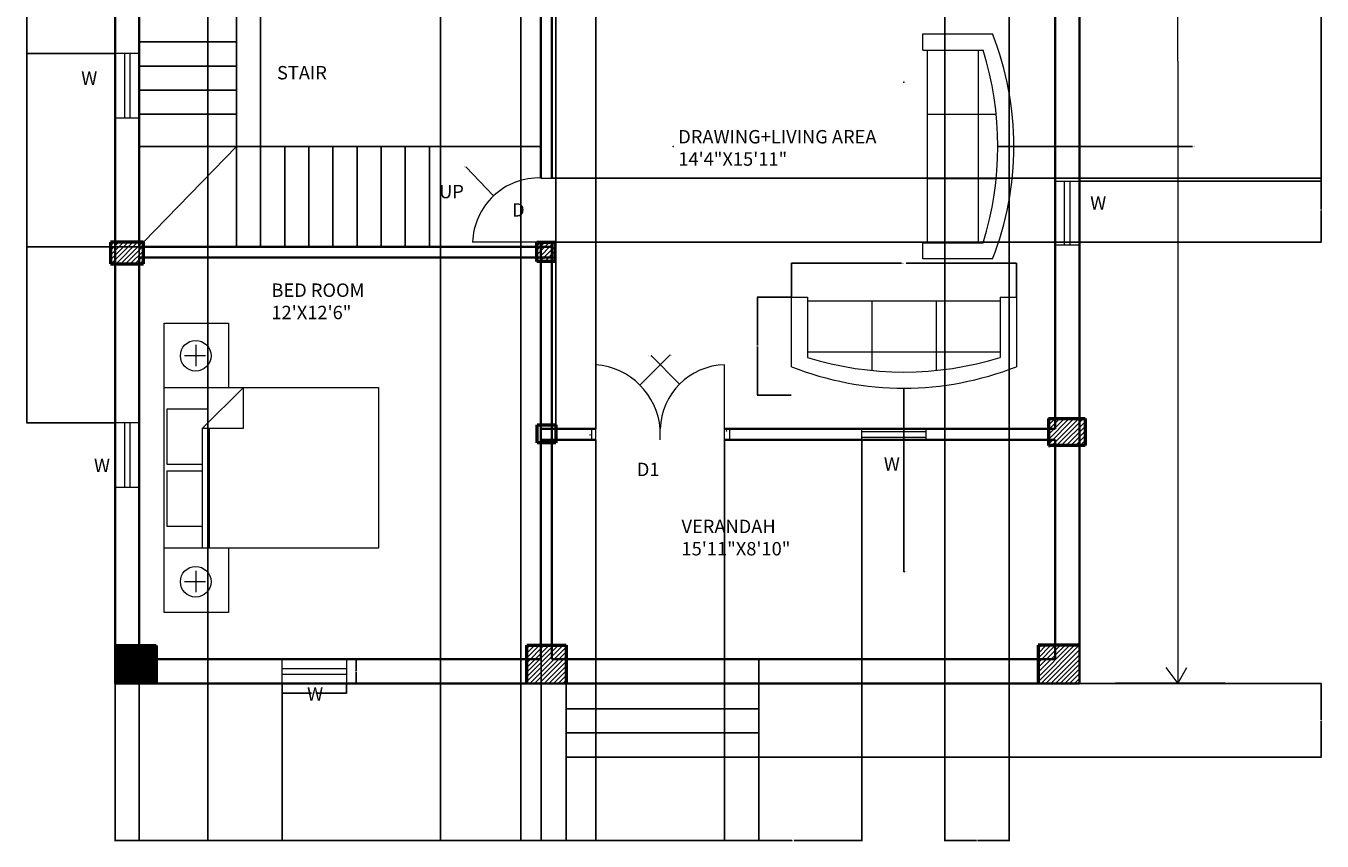
# Model space of a CAD drawing. Units: inches. Extents: x -12 to 472, y -585 to 99.
# Tile 1 of 4: x -12 to 472, y -585 to -281. Entities that reach past the tile are written whole.
import ezdxf

# ---------------------------------------------------------------- set-up
doc = ezdxf.new("R2010")
doc.units = ezdxf.units.IN
doc.header["$MEASUREMENT"] = 0
for name, color, linetype, lineweight in [('A-ANNO-DIMS', 2, 'Continuous', 18), ('A-ANNO-TEXT', 7, 'Continuous', 18), ('A-AREA-IDEN', 7, 'Continuous', 25), ('A-COLS', 7, 'Continuous', 50), ('A-COLS-PATT', 252, 'Continuous', 13), ('A-DOOR', 3, 'Continuous', 18), ('A-FLOR-STRS', 7, 'Continuous', 25), ('A-FURN', 8, 'Continuous', 18), ('A-GLAZ', 4, 'Continuous', 18), ('A-WALL', 7, 'Continuous', 35)]:
    doc.layers.add(name, color=color, linetype=linetype, lineweight=lineweight)
doc.styles.get("Standard").update_dxf_attribs({"font": 'arial.ttf'})
doc.dimstyles.get("Standard").update_dxf_attribs({"dimtxt": 0.18, "dimasz": 0.18, "dimexe": 0.18, "dimexo": 0.0625, "dimgap": 0.09, "dimtad": 0, "dimtih": 1, "dimtoh": 1, "dimdec": 4, "dimzin": 0, "dimdsep": 46, "dimtxsty": 'Standard', "dimcen": 0.09, "dimadec": 0, "dimazin": 0, "dimtfac": 1, "dimtdec": 4, "dimtofl": 0, "dimtmove": 0, "dimatfit": 3, "dimfxl": 1, "dimtolj": 1, "dimtzin": 0, "dimarcsym": 0})
pattern_1 = [(45, (-1281.9002, -702.7604), (-0.8838835, 0.8838835), [])]

# ---------------------------------------------------------------- blocks, each defined once
blk = doc.blocks.new('Bed - Queen')
for p, q in [((0, -80.00003), (0, 0)), ((0, 0), (59.99999, 0)), ((59.99999, 0), (59.99999, -80.00003)), ((7.99999, -1.2), (28.79998, -1.2)), ((7.99999, -14.4), (7.99999, -1.2)), ((28.79998, -1.2), (28.79998, -14.4)), ((31.19999, -1.2), (51.99999, -1.2)), ((31.19999, -14.4), (31.19999, -1.2)), ((51.99999, -1.2), (51.99999, -16.4)), ((0, -14.4), (44.8, -14.4)), ((59.99999, -29.6), (44.8, -14.4)), ((44.8, -14.4), (44.8, -29.6)), ((44.8, -16.8), (0, -16.8)), ((51.99999, -16.4), (46.79936, -16.4)), ((44.8, -29.6), (59.99999, -29.6)), ((59.99999, -80.00003), (0, -80.00003))]:
    blk.add_line(p, q)
blk = doc.blocks.new('Sofa - Roundback 7 ft.')
for p, q in [((-12.00002, -32.4421), (-12.00003, -6.5971)), ((11.99997, -32.4421), (11.99998, -6.5971)), ((-36.000027, -34), (-36.000027, -11.4696)), ((-35.999844, -13.3819), (35.9998, -13.3819)), ((35.99998, -34), (35.99998, -11.4696)), ((-36.000027, -32.4421), (35.99998, -32.4421))]:
    blk.add_line(p, q)
for points in [[(-36.000027, -34), (-42.000027, -34), (-42.000027, -8)], [(41.99998, -8), (41.99998, -34), (35.99998, -34)]]:
    blk.add_lwpolyline(points)
for centre, radius, start, end in [((0, -114.25), 114.25, 68.43141, 111.5686), ((-0.00001, -127.1968), 121.1968, 72.72033, 107.2797)]:
    blk.add_arc(centre, radius, start, end)
blk = doc.blocks.new('WIN-24IN-EXT')
for p, q in [((0, 5.5), (24, 5.5)), ((0, 3.5), (24, 3.5))]:
    blk.add_line(p, q)
blk.add_lwpolyline([(0, 9), (24, 9), (24, 0), (0, 0)], close=True)
blk = doc.blocks.new('NIGHTSTAND-24IN')
for p, q in [((0, 24), (24, 24)), ((24, 24), (24, 0)), ((24, 0), (0, 0))]:
    blk.add_line(p, q)
blk = doc.blocks.new('LAMP-BEDSIDE-PLAN')
for p, q in [((5.72, 9.81), (5.72, 1.79)), ((1.49, 5.8), (9.4, 5.8))]:
    blk.add_line(p, q)
blk.add_circle((5.72, 5.72), 5.72)
blk = doc.blocks.new('*D10')
at = {"layer": 'A-ANNO-DIMS', "color": 0, "lineweight": -2, "transparency": 16777216}
for p, q in [((83.68, -526.44), (83.68, -530.16)), ((107.68, -526.44), (107.68, -530.16)), ((83.86, -529.98), (94.57, -529.98)), ((107.5, -529.98), (96.8, -529.98))]:
    blk.add_line(p, q, dxfattribs=at)
at = {"layer": 'A-ANNO-DIMS', "color": 0, "transparency": 16777216}
for points in [[(83.86, -529.95), (83.86, -530.01), (83.68, -529.98)], [(107.5, -529.95), (107.5, -530.01), (107.68, -529.98)]]:
    blk.add_solid(points, dxfattribs=at)
at = {"layer": 'Defpoints', "color": 0, "transparency": 16777216}
for p in [(83.68, -526.38), (107.68, -526.38), (107.68, -529.98)]:
    blk.add_point(p, dxfattribs=at)
at = {"layer": 'A-ANNO-DIMS', "color": 0, "transparency": 16777216, "insert": (95.68, -529.98), "char_height": 0.18, "attachment_point": 5}
blk.add_mtext('\\A1;WINDOW 24 TYP.', dxfattribs=at)
blk = doc.blocks.new('*D11')
at = {"layer": 'A-ANNO-DIMS', "color": 0, "lineweight": -2, "transparency": 16777216}
for p, q in [((107.75, -517.38), (111.46, -517.38)), ((111.28, -517.56), (111.28, -521.7)), ((111.28, -526.2), (111.28, -522.06)), ((107.75, -526.38), (111.46, -526.38))]:
    blk.add_line(p, q, dxfattribs=at)
at = {"layer": 'A-ANNO-DIMS', "color": 0, "transparency": 16777216}
for points in [[(111.25, -517.56), (111.31, -517.56), (111.28, -517.38)], [(111.25, -526.2), (111.31, -526.2), (111.28, -526.38)]]:
    blk.add_solid(points, dxfattribs=at)
at = {"layer": 'Defpoints', "color": 0, "transparency": 16777216}
for p in [(107.68, -517.38), (111.28, -517.38), (107.68, -526.38)]:
    blk.add_point(p, dxfattribs=at)
at = {"layer": 'A-ANNO-DIMS', "color": 0, "transparency": 16777216, "insert": (111.28, -521.88), "char_height": 0.18, "attachment_point": 5}
blk.add_mtext('\\A1;9 TYP.', dxfattribs=at)
blk = doc.blocks.new('*D22')
at = {"layer": 'A-ANNO-DIMS', "color": 0, "lineweight": -2, "transparency": 16777216}
for p, q in [((273.76, -382.06), (273.76, -369.34)), ((273.94, -369.52), (314.86, -369.52)), ((357.58, -369.52), (316.67, -369.52)), ((357.76, -382.06), (357.76, -369.34))]:
    blk.add_line(p, q, dxfattribs=at)
at = {"layer": 'A-ANNO-DIMS', "color": 0, "transparency": 16777216}
for points in [[(273.94, -369.49), (273.94, -369.55), (273.76, -369.52)], [(357.58, -369.49), (357.58, -369.55), (357.76, -369.52)]]:
    blk.add_solid(points, dxfattribs=at)
at = {"layer": 'Defpoints', "color": 0, "transparency": 16777216}
for p in [(273.76, -369.52), (273.76, -382.12), (357.76, -382.12)]:
    blk.add_point(p, dxfattribs=at)
at = {"layer": 'A-ANNO-DIMS', "color": 0, "transparency": 16777216, "insert": (315.76, -369.52), "char_height": 0.18, "attachment_point": 5}
blk.add_mtext('\\A1;SOFA 84 TYP.', dxfattribs=at)
blk = doc.blocks.new('*D23')
at = {"layer": 'A-ANNO-DIMS', "color": 0, "lineweight": -2, "transparency": 16777216}
for p, q in [((273.7, -382.12), (260.98, -382.12)), ((261.16, -382.3), (261.16, -400.27)), ((261.16, -418.61), (261.16, -400.64)), ((273.7, -418.79), (260.98, -418.79))]:
    blk.add_line(p, q, dxfattribs=at)
at = {"layer": 'A-ANNO-DIMS', "color": 0, "transparency": 16777216}
for points in [[(261.13, -382.3), (261.19, -382.3), (261.16, -382.12)], [(261.13, -418.61), (261.19, -418.61), (261.16, -418.79)]]:
    blk.add_solid(points, dxfattribs=at)
at = {"layer": 'Defpoints', "color": 0, "transparency": 16777216}
for p in [(273.76, -382.12), (261.16, -418.79), (273.76, -418.79)]:
    blk.add_point(p, dxfattribs=at)
at = {"layer": 'A-ANNO-DIMS', "color": 0, "transparency": 16777216, "insert": (261.16, -400.46), "char_height": 0.18, "attachment_point": 5}
blk.add_mtext('\\A1;37 TYP.', dxfattribs=at)
blk = doc.blocks.new('*D26')
at = {"layer": 'A-ANNO-DIMS', "color": 0, "lineweight": -2, "transparency": 16777216}
for p, q in [((21.28, -526.44), (21.28, -585.26)), ((83.68, -526.44), (83.68, -585.26)), ((21.46, -585.08), (52.16, -585.08)), ((83.5, -585.08), (52.8, -585.08))]:
    blk.add_line(p, q, dxfattribs=at)
at = {"layer": 'A-ANNO-DIMS', "color": 0, "transparency": 16777216}
for points in [[(21.46, -585.05), (21.46, -585.11), (21.28, -585.08)], [(83.5, -585.05), (83.5, -585.11), (83.68, -585.08)]]:
    blk.add_solid(points, dxfattribs=at)
at = {"layer": 'Defpoints', "color": 0, "transparency": 16777216}
for p in [(21.28, -526.38), (83.68, -526.38), (83.68, -585.08)]:
    blk.add_point(p, dxfattribs=at)
at = {"layer": 'A-ANNO-DIMS', "color": 0, "transparency": 16777216, "insert": (52.48, -585.08), "char_height": 0.18, "attachment_point": 5}
blk.add_mtext('\\A1;62.4', dxfattribs=at)
blk = doc.blocks.new('*D27')
at = {"layer": 'A-ANNO-DIMS', "color": 0, "lineweight": -2, "transparency": 16777216}
for p, q in [((83.68, -526.44), (83.68, -585.26)), ((189.63, -553.94), (189.63, -585.26)), ((83.86, -585.08), (136.2, -585.08)), ((189.45, -585.08), (137.12, -585.08))]:
    blk.add_line(p, q, dxfattribs=at)
at = {"layer": 'A-ANNO-DIMS', "color": 0, "transparency": 16777216}
for points in [[(83.86, -585.05), (83.86, -585.11), (83.68, -585.08)], [(189.45, -585.05), (189.45, -585.11), (189.63, -585.08)]]:
    blk.add_solid(points, dxfattribs=at)
at = {"layer": 'Defpoints', "color": 0, "transparency": 16777216}
for p in [(83.68, -526.38), (189.63, -553.88), (189.63, -585.08)]:
    blk.add_point(p, dxfattribs=at)
at = {"layer": 'A-ANNO-DIMS', "color": 0, "transparency": 16777216, "insert": (136.66, -585.08), "char_height": 0.18, "attachment_point": 5}
blk.add_mtext('\\A1;105.95', dxfattribs=at)
blk = doc.blocks.new('*D28')
at = {"layer": 'A-ANNO-DIMS', "color": 0, "lineweight": -2, "transparency": 16777216}
for p, q in [((189.63, -553.94), (189.63, -585.26)), ((261.62, -553.94), (261.62, -585.26)), ((189.81, -585.08), (225.23, -585.08)), ((261.44, -585.08), (226.02, -585.08))]:
    blk.add_line(p, q, dxfattribs=at)
at = {"layer": 'A-ANNO-DIMS', "color": 0, "transparency": 16777216}
for points in [[(189.81, -585.05), (189.81, -585.11), (189.63, -585.08)], [(261.44, -585.05), (261.44, -585.11), (261.62, -585.08)]]:
    blk.add_solid(points, dxfattribs=at)
at = {"layer": 'Defpoints', "color": 0, "transparency": 16777216}
for p in [(189.63, -553.88), (261.62, -553.88), (261.62, -585.08)]:
    blk.add_point(p, dxfattribs=at)
at = {"layer": 'A-ANNO-DIMS', "color": 0, "transparency": 16777216, "insert": (225.63, -585.08), "char_height": 0.18, "attachment_point": 5}
blk.add_mtext('\\A1;71.98', dxfattribs=at)
blk = doc.blocks.new('*D29')
at = {"layer": 'A-ANNO-DIMS', "color": 0, "lineweight": -2, "transparency": 16777216}
for p, q in [((381.34, -526.38), (471.69, -526.38)), ((471.51, -526.56), (471.51, -539.95)), ((471.51, -553.7), (471.51, -540.31)), ((261.68, -553.88), (471.69, -553.88))]:
    blk.add_line(p, q, dxfattribs=at)
at = {"layer": 'A-ANNO-DIMS', "color": 0, "transparency": 16777216}
for points in [[(471.48, -526.56), (471.54, -526.56), (471.51, -526.38)], [(471.48, -553.7), (471.54, -553.7), (471.51, -553.88)]]:
    blk.add_solid(points, dxfattribs=at)
at = {"layer": 'Defpoints', "color": 0, "transparency": 16777216}
for p in [(381.28, -526.38), (471.51, -526.38), (261.62, -553.88)]:
    blk.add_point(p, dxfattribs=at)
at = {"layer": 'A-ANNO-DIMS', "color": 0, "transparency": 16777216, "insert": (471.51, -540.13), "char_height": 0.18, "attachment_point": 5}
blk.add_mtext('\\A1;27.5', dxfattribs=at)
blk = doc.blocks.new('*D30')
at = {"layer": 'A-ANNO-DIMS', "color": 0, "lineweight": -2, "transparency": 16777216}
for p, q in [((185.8, -429.83), (185.8, 98.81)), ((185.98, 98.63), (193.09, 98.63)), ((200.62, 98.63), (193.51, 98.63)), ((200.8, -431.32), (200.8, 98.81))]:
    blk.add_line(p, q, dxfattribs=at)
at = {"layer": 'A-ANNO-DIMS', "color": 0, "transparency": 16777216}
for points in [[(185.98, 98.66), (185.98, 98.6), (185.8, 98.63)], [(200.62, 98.66), (200.62, 98.6), (200.8, 98.63)]]:
    blk.add_solid(points, dxfattribs=at)
at = {"layer": 'Defpoints', "color": 0, "transparency": 16777216}
for p in [(200.8, 98.63), (185.8, -429.9), (200.8, -431.38)]:
    blk.add_point(p, dxfattribs=at)
at = {"layer": 'A-ANNO-DIMS', "color": 0, "transparency": 16777216, "insert": (193.3, 98.63), "char_height": 0.18, "attachment_point": 5}
blk.add_mtext('\\A1;15', dxfattribs=at)
blk = doc.blocks.new('*D31')
at = {"layer": 'A-ANNO-DIMS', "color": 0, "lineweight": -2, "transparency": 16777216}
for p, q in [((200.8, -435.44), (200.8, -585.26)), ((248.8, -435.44), (248.8, -585.26)), ((200.98, -585.08), (224.58, -585.08)), ((248.62, -585.08), (225.03, -585.08))]:
    blk.add_line(p, q, dxfattribs=at)
at = {"layer": 'A-ANNO-DIMS', "color": 0, "transparency": 16777216}
for points in [[(200.98, -585.05), (200.98, -585.11), (200.8, -585.08)], [(248.62, -585.05), (248.62, -585.11), (248.8, -585.08)]]:
    blk.add_solid(points, dxfattribs=at)
at = {"layer": 'Defpoints', "color": 0, "transparency": 16777216}
for p in [(200.8, -435.38), (248.8, -435.38), (248.8, -585.08)]:
    blk.add_point(p, dxfattribs=at)
at = {"layer": 'A-ANNO-DIMS', "color": 0, "transparency": 16777216, "insert": (224.8, -585.08), "char_height": 0.18, "attachment_point": 5}
blk.add_mtext('\\A1;48', dxfattribs=at)
blk = doc.blocks.new('*D32')
at = {"layer": 'A-ANNO-DIMS', "color": 0, "lineweight": -2, "transparency": 16777216}
for p, q in [((248.8, -435.44), (248.8, -585.26)), ((300, -435.44), (300, -585.26)), ((248.98, -585.08), (274.01, -585.08)), ((299.82, -585.08), (274.79, -585.08))]:
    blk.add_line(p, q, dxfattribs=at)
at = {"layer": 'A-ANNO-DIMS', "color": 0, "transparency": 16777216}
for points in [[(248.98, -585.05), (248.98, -585.11), (248.8, -585.08)], [(299.82, -585.05), (299.82, -585.11), (300, -585.08)]]:
    blk.add_solid(points, dxfattribs=at)
at = {"layer": 'Defpoints', "color": 0, "transparency": 16777216}
for p in [(248.8, -435.38), (300, -435.38), (300, -585.08)]:
    blk.add_point(p, dxfattribs=at)
at = {"layer": 'A-ANNO-DIMS', "color": 0, "transparency": 16777216, "insert": (274.4, -585.08), "char_height": 0.18, "attachment_point": 5}
blk.add_mtext('\\A1;51.19', dxfattribs=at)
blk = doc.blocks.new('*D33')
at = {"layer": 'A-ANNO-DIMS', "color": 0, "lineweight": -2, "transparency": 16777216}
for p, q in [((30.28, -363.44), (30.28, -585.26)), ((180.28, -363.44), (180.28, -585.26)), ((30.46, -585.08), (105, -585.08)), ((180.1, -585.08), (105.56, -585.08))]:
    blk.add_line(p, q, dxfattribs=at)
at = {"layer": 'A-ANNO-DIMS', "color": 0, "transparency": 16777216}
for points in [[(30.46, -585.05), (30.46, -585.11), (30.28, -585.08)], [(180.1, -585.05), (180.1, -585.11), (180.28, -585.08)]]:
    blk.add_solid(points, dxfattribs=at)
at = {"layer": 'Defpoints', "color": 0, "transparency": 16777216}
for p in [(30.28, -363.38), (180.28, -363.38), (180.28, -585.08)]:
    blk.add_point(p, dxfattribs=at)
at = {"layer": 'A-ANNO-DIMS', "color": 0, "transparency": 16777216, "insert": (105.28, -585.08), "char_height": 0.18, "attachment_point": 5}
blk.add_mtext('\\A1;150', dxfattribs=at)
blk = doc.blocks.new('*D34')
at = {"layer": 'A-ANNO-DIMS', "color": 0, "lineweight": -2, "transparency": 16777216}
for p, q in [((30.22, -240.38), (-11.82, -240.38)), ((-11.64, -240.56), (-11.64, -301.7)), ((-11.64, -363.2), (-11.64, -302.06)), ((30.22, -363.38), (-11.82, -363.38))]:
    blk.add_line(p, q, dxfattribs=at)
at = {"layer": 'A-ANNO-DIMS', "color": 0, "transparency": 16777216}
for points in [[(-11.67, -240.56), (-11.61, -240.56), (-11.64, -240.38)], [(-11.67, -363.2), (-11.61, -363.2), (-11.64, -363.38)]]:
    blk.add_solid(points, dxfattribs=at)
at = {"layer": 'Defpoints', "color": 0, "transparency": 16777216}
for p in [(30.28, -240.38), (-11.64, -363.38), (30.28, -363.38)]:
    blk.add_point(p, dxfattribs=at)
at = {"layer": 'A-ANNO-DIMS', "color": 0, "transparency": 16777216, "insert": (-11.64, -301.88), "char_height": 0.18, "attachment_point": 5}
blk.add_mtext('\\A1;123', dxfattribs=at)
blk = doc.blocks.new('*D35')
at = {"layer": 'A-ANNO-DIMS', "color": 0, "lineweight": -2, "transparency": 16777216}
for p, q in [((30.28, -325.82), (30.28, 98.81)), ((30.46, 98.63), (47.98, 98.63)), ((66.43, 98.63), (48.91, 98.63)), ((66.61, -325.82), (66.61, 98.81))]:
    blk.add_line(p, q, dxfattribs=at)
at = {"layer": 'A-ANNO-DIMS', "color": 0, "transparency": 16777216}
for points in [[(30.46, 98.66), (30.46, 98.6), (30.28, 98.63)], [(66.43, 98.66), (66.43, 98.6), (66.61, 98.63)]]:
    blk.add_solid(points, dxfattribs=at)
at = {"layer": 'Defpoints', "color": 0, "transparency": 16777216}
for p in [(66.61, 98.63), (30.28, -325.88), (66.61, -325.88)]:
    blk.add_point(p, dxfattribs=at)
at = {"layer": 'A-ANNO-DIMS', "color": 0, "transparency": 16777216, "insert": (48.45, 98.63), "char_height": 0.18, "attachment_point": 5}
blk.add_mtext('\\A1;36.335', dxfattribs=at)
blk = doc.blocks.new('*D36')
at = {"layer": 'A-ANNO-DIMS', "color": 0, "lineweight": -2, "transparency": 16777216}
for p, q in [((66.61, -325.82), (66.61, 98.81)), ((66.79, 98.63), (70.96, 98.63)), ((75.43, 98.63), (71.26, 98.63)), ((75.61, -325.82), (75.61, 98.81))]:
    blk.add_line(p, q, dxfattribs=at)
at = {"layer": 'A-ANNO-DIMS', "color": 0, "transparency": 16777216}
for points in [[(66.79, 98.66), (66.79, 98.6), (66.61, 98.63)], [(75.43, 98.66), (75.43, 98.6), (75.61, 98.63)]]:
    blk.add_solid(points, dxfattribs=at)
at = {"layer": 'Defpoints', "color": 0, "transparency": 16777216}
for p in [(75.61, 98.63), (66.61, -325.88), (75.61, -325.88)]:
    blk.add_point(p, dxfattribs=at)
at = {"layer": 'A-ANNO-DIMS', "color": 0, "transparency": 16777216, "insert": (71.11, 98.63), "char_height": 0.18, "attachment_point": 5}
blk.add_mtext('\\A1;9', dxfattribs=at)
blk = doc.blocks.new('*D38')
at = {"layer": 'A-ANNO-DIMS', "color": 0, "lineweight": -2, "transparency": 16777216}
for p, q in [((184.34, -337.67), (471.69, -337.67)), ((471.51, -337.85), (471.51, -349.49)), ((471.51, -361.49), (471.51, -349.85)), ((178.82, -361.67), (471.69, -361.67))]:
    blk.add_line(p, q, dxfattribs=at)
at = {"layer": 'A-ANNO-DIMS', "color": 0, "transparency": 16777216}
for points in [[(471.48, -337.85), (471.54, -337.85), (471.51, -337.67)], [(471.48, -361.49), (471.54, -361.49), (471.51, -361.67)]]:
    blk.add_solid(points, dxfattribs=at)
at = {"layer": 'Defpoints', "color": 0, "transparency": 16777216}
for p in [(184.28, -337.67), (178.76, -361.67), (471.51, -361.67)]:
    blk.add_point(p, dxfattribs=at)
at = {"layer": 'A-ANNO-DIMS', "color": 0, "transparency": 16777216, "insert": (471.51, -349.67), "char_height": 0.18, "attachment_point": 5}
blk.add_mtext('\\A1;24', dxfattribs=at)
blk = doc.blocks.new('*D39')
at = {"layer": 'A-ANNO-DIMS', "color": 0, "lineweight": -2, "transparency": 16777216}
for p, q in [((142.75, -137.44), (142.75, -585.26)), ((172.75, -137.44), (172.75, -585.26)), ((142.93, -585.08), (157.53, -585.08)), ((172.57, -585.08), (157.97, -585.08))]:
    blk.add_line(p, q, dxfattribs=at)
at = {"layer": 'A-ANNO-DIMS', "color": 0, "transparency": 16777216}
for points in [[(142.93, -585.05), (142.93, -585.11), (142.75, -585.08)], [(172.57, -585.05), (172.57, -585.11), (172.75, -585.08)]]:
    blk.add_solid(points, dxfattribs=at)
at = {"layer": 'Defpoints', "color": 0, "transparency": 16777216}
for p in [(142.75, -137.38), (172.75, -137.38), (172.75, -585.08)]:
    blk.add_point(p, dxfattribs=at)
at = {"layer": 'A-ANNO-DIMS', "color": 0, "transparency": 16777216, "insert": (157.75, -585.08), "char_height": 0.18, "attachment_point": 5}
blk.add_mtext('\\A1;30', dxfattribs=at)
blk = doc.blocks.new('*D40')
at = {"layer": 'A-ANNO-DIMS', "color": 0, "lineweight": -2, "transparency": 16777216}
for p, q in [((331.04, -77.44), (331.04, -585.26)), ((355.04, -77.44), (355.04, -585.26)), ((331.22, -585.08), (342.82, -585.08)), ((354.86, -585.08), (343.26, -585.08))]:
    blk.add_line(p, q, dxfattribs=at)
at = {"layer": 'A-ANNO-DIMS', "color": 0, "transparency": 16777216}
for points in [[(331.22, -585.05), (331.22, -585.11), (331.04, -585.08)], [(354.86, -585.05), (354.86, -585.11), (355.04, -585.08)]]:
    blk.add_solid(points, dxfattribs=at)
at = {"layer": 'Defpoints', "color": 0, "transparency": 16777216}
for p in [(331.04, -77.38), (355.04, -77.38), (355.04, -585.08)]:
    blk.add_point(p, dxfattribs=at)
at = {"layer": 'A-ANNO-DIMS', "color": 0, "transparency": 16777216, "insert": (343.04, -585.08), "char_height": 0.18, "attachment_point": 5}
blk.add_mtext('\\A1;24', dxfattribs=at)
blk = doc.blocks.new('*D44')
at = {"layer": 'A-ANNO-DIMS', "color": 0, "lineweight": -2, "transparency": 16777216}
for p, q in [((30.28, -137.44), (30.28, -585.26)), ((55.95, -137.44), (55.95, -585.26)), ((30.46, -585.08), (42.65, -585.08)), ((55.77, -585.08), (43.58, -585.08))]:
    blk.add_line(p, q, dxfattribs=at)
at = {"layer": 'A-ANNO-DIMS', "color": 0, "transparency": 16777216}
for points in [[(30.46, -585.05), (30.46, -585.11), (30.28, -585.08)], [(55.77, -585.05), (55.77, -585.11), (55.95, -585.08)]]:
    blk.add_solid(points, dxfattribs=at)
at = {"layer": 'Defpoints', "color": 0, "transparency": 16777216}
for p in [(30.28, -137.38), (55.95, -137.38), (55.95, -585.08)]:
    blk.add_point(p, dxfattribs=at)
at = {"layer": 'A-ANNO-DIMS', "color": 0, "transparency": 16777216, "insert": (43.12, -585.08), "char_height": 0.18, "attachment_point": 5}
blk.add_mtext('\\A1;25.674', dxfattribs=at)
blk = doc.blocks.new('*D48')
at = {"layer": 'A-ANNO-DIMS', "color": 0, "lineweight": -2, "transparency": 16777216}
for p, q in [((21.22, -171.85), (-11.82, -171.85)), ((-11.64, -172.03), (-11.64, -231.32)), ((-11.64, -290.98), (-11.64, -231.69)), ((21.22, -291.16), (-11.82, -291.16))]:
    blk.add_line(p, q, dxfattribs=at)
at = {"layer": 'A-ANNO-DIMS', "color": 0, "transparency": 16777216}
for points in [[(-11.67, -172.03), (-11.61, -172.03), (-11.64, -171.85)], [(-11.67, -290.98), (-11.61, -290.98), (-11.64, -291.16)]]:
    blk.add_solid(points, dxfattribs=at)
at = {"layer": 'Defpoints', "color": 0, "transparency": 16777216}
for p in [(21.28, -171.85), (-11.64, -291.16), (21.28, -291.16)]:
    blk.add_point(p, dxfattribs=at)
at = {"layer": 'A-ANNO-DIMS', "color": 0, "transparency": 16777216, "insert": (-11.64, -231.51), "char_height": 0.18, "attachment_point": 5}
blk.add_mtext('\\A1;119.3', dxfattribs=at)
blk = doc.blocks.new('*D49')
at = {"layer": 'A-ANNO-DIMS', "color": 0, "lineweight": -2, "transparency": 16777216}
for p, q in [((21.22, -291.16), (-11.82, -291.16)), ((-11.64, -291.34), (-11.64, -359.95)), ((-11.64, -428.93), (-11.64, -360.32)), ((21.22, -429.11), (-11.82, -429.11))]:
    blk.add_line(p, q, dxfattribs=at)
at = {"layer": 'A-ANNO-DIMS', "color": 0, "transparency": 16777216}
for points in [[(-11.67, -291.34), (-11.61, -291.34), (-11.64, -291.16)], [(-11.67, -428.93), (-11.61, -428.93), (-11.64, -429.11)]]:
    blk.add_solid(points, dxfattribs=at)
at = {"layer": 'Defpoints', "color": 0, "transparency": 16777216}
for p in [(21.28, -291.16), (-11.64, -429.11), (21.28, -429.11)]:
    blk.add_point(p, dxfattribs=at)
at = {"layer": 'A-ANNO-DIMS', "color": 0, "transparency": 16777216, "insert": (-11.64, -360.13), "char_height": 0.18, "attachment_point": 5}
blk.add_mtext('\\A1;137.95', dxfattribs=at)
blk = doc.blocks.new('*D51')
at = {"layer": 'A-ANNO-DIMS', "color": 0, "lineweight": -2, "transparency": 16777216}
for p, q in [((381.34, -186.88), (471.69, -186.88)), ((471.51, -187.06), (471.51, -262.66)), ((471.51, -338.62), (471.51, -263.02)), ((381.34, -338.8), (471.69, -338.8))]:
    blk.add_line(p, q, dxfattribs=at)
at = {"layer": 'A-ANNO-DIMS', "color": 0, "transparency": 16777216}
for points in [[(471.48, -187.06), (471.54, -187.06), (471.51, -186.88)], [(471.48, -338.62), (471.54, -338.62), (471.51, -338.8)]]:
    blk.add_solid(points, dxfattribs=at)
at = {"layer": 'Defpoints', "color": 0, "transparency": 16777216}
for p in [(381.28, -186.88), (381.28, -338.8), (471.51, -338.8)]:
    blk.add_point(p, dxfattribs=at)
at = {"layer": 'A-ANNO-DIMS', "color": 0, "transparency": 16777216, "insert": (471.51, -262.84), "char_height": 0.18, "attachment_point": 5}
blk.add_mtext('\\A1;151.92', dxfattribs=at)
blk = doc.blocks.new('*D52')
at = {"layer": 'A-ANNO-DIMS', "color": 0, "lineweight": -2, "transparency": 16777216}
for p, q in [((228.35, -403.83), (217.32, -414.87)), ((228.53, -403.83), (228.35, -403.83)), ((198.49, -433.6), (198.67, -433.6)), ((198.58, -433.69), (198.58, -433.51))]:
    blk.add_line(p, q, dxfattribs=at)
at = {"layer": 'A-ANNO-DIMS', "color": 0, "transparency": 16777216}
blk.add_solid([(217.29, -414.84), (217.34, -414.89), (217.19, -414.99)], dxfattribs=at)
at = {"layer": 'Defpoints', "color": 0, "transparency": 16777216}
for p in [(217.19, -414.99), (198.58, -433.6)]:
    blk.add_point(p, dxfattribs=at)
at = {"layer": 'A-ANNO-DIMS', "color": 0, "transparency": 16777216, "insert": (229.01, -403.83), "char_height": 0.18, "attachment_point": 5}
blk.add_mtext('\\A1;R26.32', dxfattribs=at)
blk = doc.blocks.new('*D53')
at = {"layer": 'A-ANNO-DIMS', "color": 0, "lineweight": -2, "transparency": 16777216}
for p, q in [((221.36, -404.12), (221.54, -404.12)), ((221.54, -404.12), (231.91, -414.49)), ((249.45, -432.12), (249.63, -432.12)), ((249.54, -432.21), (249.54, -432.03))]:
    blk.add_line(p, q, dxfattribs=at)
at = {"layer": 'A-ANNO-DIMS', "color": 0, "transparency": 16777216}
blk.add_solid([(231.93, -414.47), (231.89, -414.51), (232.04, -414.62)], dxfattribs=at)
at = {"layer": 'Defpoints', "color": 0, "transparency": 16777216}
for p in [(232.04, -414.62), (249.54, -432.12)]:
    blk.add_point(p, dxfattribs=at)
at = {"layer": 'A-ANNO-DIMS', "color": 0, "transparency": 16777216, "insert": (220.88, -404.12), "char_height": 0.18, "attachment_point": 5}
blk.add_mtext('\\A1;R24.75', dxfattribs=at)
blk = doc.blocks.new('*D54')
at = {"layer": 'A-ANNO-DIMS', "color": 0, "lineweight": -2, "transparency": 16777216}
for p, q in [((152.19, -333.57), (152.37, -333.57)), ((152.37, -333.57), (162.4, -344.23)), ((179.35, -362.36), (179.53, -362.36)), ((179.44, -362.45), (179.44, -362.27))]:
    blk.add_line(p, q, dxfattribs=at)
at = {"layer": 'A-ANNO-DIMS', "color": 0, "transparency": 16777216}
blk.add_solid([(162.42, -344.21), (162.38, -344.25), (162.52, -344.36)], dxfattribs=at)
at = {"layer": 'Defpoints', "color": 0, "transparency": 16777216}
for p in [(162.52, -344.36), (179.44, -362.36)]:
    blk.add_point(p, dxfattribs=at)
at = {"layer": 'A-ANNO-DIMS', "color": 0, "transparency": 16777216, "insert": (151.78, -333.57), "char_height": 0.18, "attachment_point": 5}
blk.add_mtext('\\A1;R24.7', dxfattribs=at)
blk = doc.blocks.new('*D60')
at = {"layer": 'A-ANNO-DIMS', "color": 0, "lineweight": -2, "transparency": 16777216}
for p, q in [((229.56, -325.88), (229.74, -325.88)), ((229.65, -325.97), (229.65, -325.79)), ((423.56, -325.88), (351.03, -325.88))]:
    blk.add_line(p, q, dxfattribs=at)
at = {"layer": 'A-ANNO-DIMS', "color": 0, "transparency": 16777216}
blk.add_solid([(351.03, -325.85), (351.03, -325.91), (350.85, -325.88)], dxfattribs=at)
at = {"layer": 'Defpoints', "color": 0, "transparency": 16777216}
for p in [(229.65, -325.88), (350.85, -325.88)]:
    blk.add_point(p, dxfattribs=at)
at = {"layer": 'A-ANNO-DIMS', "color": 0, "transparency": 16777216, "insert": (424.24, -325.88), "char_height": 0.18, "attachment_point": 5}
blk.add_mtext('\\A1;2X R121.2', dxfattribs=at)
blk = doc.blocks.new('*D61')
at = {"layer": 'A-ANNO-DIMS', "color": 0, "lineweight": -2, "transparency": 16777216}
for p, q in [((315.67, -301.87), (315.85, -301.87)), ((315.76, -301.96), (315.76, -301.78)), ((315.76, -484.67), (315.76, -416.3)), ((315.94, -484.67), (315.76, -484.67))]:
    blk.add_line(p, q, dxfattribs=at)
at = {"layer": 'A-ANNO-DIMS', "color": 0, "transparency": 16777216}
blk.add_solid([(315.79, -416.3), (315.73, -416.3), (315.76, -416.12)], dxfattribs=at)
at = {"layer": 'Defpoints', "color": 0, "transparency": 16777216}
for p in [(315.76, -301.87), (315.76, -416.12)]:
    blk.add_point(p, dxfattribs=at)
at = {"layer": 'A-ANNO-DIMS', "color": 0, "transparency": 16777216, "insert": (316.69, -484.67), "char_height": 0.18, "attachment_point": 5}
blk.add_mtext('\\A1;2X R114.25', dxfattribs=at)

msp = doc.modelspace()

# ---------------------------------------------------------------- hatches: boundary and pattern name
at = {"layer": 'A-COLS-PATT'}
h = msp.add_hatch(dxfattribs=at)
h.set_pattern_fill('ANSI31', color=256, scale=10)
h.set_pattern_definition(pattern_1)
h.paths.add_polyline_path([(184.2783, -361.6735), (180.2783, -361.6735), (180.2783, -363.3788), (184.2783, -363.3788)])
h.paths.add_polyline_path([(184.2783, -363.3788), (180.2783, -363.3788), (180.2783, -367.3788), (184.2783, -367.3788)])
h.paths.add_polyline_path([(180.2783, -363.3788), (178.7557, -363.3788), (178.7557, -367.3788), (180.2783, -367.3788)])
h.paths.add_polyline_path([(180.2783, -361.6735), (178.7557, -361.6735), (178.7557, -363.3788), (180.2783, -363.3788)])
h.paths.add_polyline_path([(185.4517, -361.6735), (184.2783, -361.6735), (184.2783, -363.3788), (184.2783, -367.3788), (184.2783, -368.8013), (185.4517, -368.8013)])
h.paths.add_polyline_path([(184.2783, -367.3788), (180.2783, -367.3788), (180.2783, -368.8013), (184.2783, -368.8013)])
h.paths.add_polyline_path([(180.2783, -367.3788), (178.7557, -367.3788), (178.7557, -368.8013), (180.2783, -368.8013)])
h.paths.add_polyline_path([(31.8418, -363.3788), (30.2783, -363.3788), (30.2783, -361.6831), (21.2783, -361.6831), (21.2783, -369.7536), (30.2783, -369.7536), (30.2783, -367.3788), (31.8418, -367.3788)])
h.paths.add_polyline_path([(21.2783, -361.6831), (19.5559, -361.6831), (19.5559, -369.7536), (21.2783, -369.7536)])
h.paths.add_polyline_path([(31.8418, -361.6831), (31.7311, -361.6831), (30.2783, -361.6831), (30.2783, -363.3788), (31.8418, -363.3788)], flags=17)
h.paths.add_polyline_path([(31.8418, -367.3788), (30.2783, -367.3788), (30.2783, -369.7536), (31.8418, -369.7536)], flags=17)
h = msp.add_hatch(dxfattribs=at)
h.set_pattern_fill('ANSI31', color=256, scale=10)
h.set_pattern_definition(pattern_1)
h.paths.add_polyline_path([(381.2783, -427.5256), (372.2783, -427.5256), (372.2783, -431.3788), (369.7477, -431.3788), (369.7477, -435.3788), (372.2783, -435.3788), (372.2783, -437.5759), (381.2783, -437.5759)])
h.paths.add_polyline_path([(383.4388, -427.5256), (381.2783, -427.5256), (381.2783, -437.5759), (383.4388, -437.5759)])
h.paths.add_polyline_path([(372.2783, -427.5256), (369.7477, -427.5256), (369.7477, -431.3788), (372.2783, -431.3788)], flags=17)
h.paths.add_polyline_path([(372.2783, -435.3788), (369.7477, -435.3788), (369.7477, -437.5759), (370.4076, -437.5759), (372.2783, -437.5759)])
h.paths.add_polyline_path([(372.2783, -512.16), (365.8725, -512.16), (365.8725, -517.3788), (372.2783, -517.3788)], flags=17)
h.paths.add_polyline_path([(381.2783, -512.16), (372.2783, -512.16), (372.2783, -517.3788), (365.8725, -517.3788), (365.8725, -526.3788), (381.2783, -526.3788)])
h = msp.add_hatch(dxfattribs=at)
h.set_pattern_fill('ANSI31', color=256, scale=3.5)
h.set_pattern_definition([(45, (-1281.90016, -702.76037), (-0.30935922, 0.30935922), [])])
h.paths.add_polyline_path([(36.6123, -512.2155), (30.2783, -512.2155), (30.2783, -517.3788), (36.6123, -517.3788)], flags=17)
h.paths.add_polyline_path([(36.6123, -517.3788), (30.2783, -517.3788), (30.2783, -512.2155), (21.2783, -512.2155), (21.2783, -526.3788), (36.6123, -526.3788)])
h = msp.add_hatch(dxfattribs=at)
h.set_pattern_fill('ANSI31', color=256, scale=10)
h.set_pattern_definition(pattern_1)
h.paths.add_polyline_path([(189.6349, -517.3788), (184.2783, -517.3788), (184.2783, -512.1371), (180.2783, -512.1371), (180.2783, -517.3788), (175.0056, -517.3788), (175.0056, -526.3788), (189.6349, -526.3788)])
h.paths.add_polyline_path([(180.2783, -512.1371), (175.0056, -512.1371), (175.0056, -517.3788), (180.2783, -517.3788)], flags=17)
h.paths.add_polyline_path([(189.6349, -512.1371), (184.2783, -512.1371), (184.2783, -517.3788), (189.6349, -517.3788)], flags=17)

# ---------------------------------------------------------------- linework, layer by layer
at = {"layer": 'A-ANNO-DIMS'}
for p, q in [((417.9974, -293.9965), (417.9974, -272.3584)), ((417.9974, -293.9965), (417.9974, -526.3788)), ((413.5001, -520.5042), (417.9974, -526.3788)), ((417.9974, -526.3788), (421.4306, -520.4322)), ((394.7437, -526.1467), (435.612, -526.1467))]:
    msp.add_line(p, q, dxfattribs=at)
at = {"layer": 'A-COLS'}
for p, q in [((31.7311, -361.6831), (19.5559, -361.6831)), ((19.5559, -361.6831), (19.5559, -369.7536)), ((31.7311, -361.6831), (31.8418, -361.6831)), ((31.8418, -369.7536), (31.8418, -361.6831)), ((178.7557, -361.6735), (185.4517, -361.6735)), ((178.7557, -368.8013), (178.7557, -361.6735)), ((185.4517, -361.6735), (185.4517, -368.8013)), ((19.5559, -369.7536), (31.8418, -369.7536)), ((185.4517, -368.8013), (178.7557, -368.8013)), ((178.9047, -429.897), (185.8034, -429.897)), ((178.9047, -436.5724), (178.9047, -429.897)), ((185.8034, -429.897), (185.8034, -436.5724)), ((369.7477, -427.5256), (383.4388, -427.5256)), ((369.7477, -427.5256), (369.7477, -437.5759)), ((383.4388, -427.5256), (383.4388, -437.5759)), ((185.8034, -436.5724), (178.9047, -436.5724)), ((369.7477, -437.5759), (370.4076, -437.5759)), ((383.4388, -437.5759), (370.4076, -437.5759)), ((21.2783, -512.2155), (36.6123, -512.2155)), ((36.6123, -512.2155), (36.6123, -526.3788)), ((175.0056, -526.3788), (175.0056, -512.1371)), ((175.0056, -512.1371), (189.6349, -512.1371)), ((189.6349, -512.1371), (189.6349, -526.3788)), ((381.2783, -512.16), (365.8725, -512.16)), ((365.8725, -512.16), (365.8725, -526.3788))]:
    msp.add_line(p, q, dxfattribs=at)
at = {"layer": 'A-DOOR'}
for p, q in [((180.2783, -337.6735), (184.2783, -337.6735)), ((178.7557, -361.6735), (154.7557, -361.6735)), ((200.803, -431.3788), (200.803, -407.3788)), ((248.803, -431.3788), (248.803, -407.3788)), ((199.186, -431.3788), (199.186, -435.3788)), ((200.803, -435.3788), (200.803, -431.3788)), ((224.803, -435.3788), (224.803, -431.3788)), ((248.803, -435.3788), (248.803, -431.3788)), ((250.6168, -431.3788), (250.6168, -435.3788))]:
    msp.add_line(p, q, dxfattribs=at)
for centre, radius, start, end in [((179.4439, -362.357), 24.6977, 88.063909, 178.414032), ((198.5782, -433.6035), 26.3189, 4.849003, 85.150997), ((249.5412, -432.117), 24.7493, 91.709347, 178.290653)]:
    msp.add_arc(centre, radius, start, end, dxfattribs=at)
at = {"layer": 'A-FLOR-STRS'}
for p, q in [((66.6133, -240.3222), (66.6133, -363.3788)), ((30.2783, -286.8788), (66.6133, -286.8788)), ((30.2783, -295.8788), (66.6133, -295.8788)), ((30.2783, -304.8788), (66.6133, -304.8788)), ((30.2783, -313.8788), (66.6133, -313.8788)), ((30.2783, -325.8788), (180.2783, -325.8788)), ((31.8418, -361.6831), (66.6133, -325.8788)), ((75.6133, -325.8788), (75.6133, -363.3788)), ((84.6133, -325.8788), (84.6133, -363.3788)), ((93.6133, -325.8788), (93.6133, -363.3788)), ((102.6133, -325.8788), (102.6133, -363.3788)), ((111.6133, -325.8788), (111.6133, -363.3788)), ((120.6133, -325.8788), (120.6133, -363.3788)), ((129.6133, -325.8788), (129.6133, -363.3788)), ((138.6133, -325.8788), (138.6133, -363.3788)), ((261.6165, -553.8813), (261.6165, -517.3788)), ((189.6349, -526.3788), (189.6349, -553.8813)), ((189.6349, -535.8813), (245.6443, -535.8813)), ((245.6443, -535.8813), (261.6165, -535.8813)), ((189.6349, -544.8813), (245.6443, -544.8813)), ((245.6443, -544.8813), (261.6165, -544.8813)), ((189.6349, -553.8813), (245.6443, -553.8813)), ((245.6443, -553.8813), (261.6165, -553.8813))]:
    msp.add_line(p, q, dxfattribs=at)
at = {"layer": 'A-GLAZ'}
for p, q in [((299.9961, -432.3788), (323.9961, -432.3788)), ((299.9961, -432.3788), (323.9961, -432.3788)), ((299.9961, -434.3788), (323.9961, -434.3788))]:
    msp.add_line(p, q, dxfattribs=at)
msp.add_lwpolyline([(299.9961, -431.3788), (323.9961, -431.3788), (323.9961, -435.3788), (299.9961, -435.3788)], close=True, dxfattribs=at)
at = {"layer": 'A-WALL'}
for p, q in [((180.2783, -337.6735), (180.2783, -236.3788)), ((184.2783, -337.6735), (184.2783, -236.3788)), ((30.2783, -363.3788), (30.2783, -240.3788)), ((372.2783, -240.3788), (372.2783, -431.3788)), ((180.2783, -363.3788), (180.2783, -361.6735)), ((184.2783, -363.3788), (184.2783, -361.6735)), ((184.2783, -363.3788), (30.2783, -363.3788)), ((30.2783, -517.3788), (30.2783, -367.3788)), ((184.2783, -367.3788), (30.2783, -367.3788)), ((180.2783, -517.3788), (180.2783, -363.3788)), ((184.2783, -517.3788), (184.2783, -363.3788)), ((180.2783, -431.3788), (200.803, -431.3788)), ((180.2783, -435.3788), (200.803, -435.3788)), ((248.803, -431.3788), (372.2783, -431.3788)), ((248.803, -435.3788), (372.2783, -435.3788)), ((372.2783, -435.3788), (372.2783, -517.3788)), ((180.2783, -517.3788), (30.2783, -517.3788)), ((372.2783, -517.3788), (184.2783, -517.3788))]:
    msp.add_line(p, q, dxfattribs=at)
msp.add_lwpolyline([(21.2783, 19.6212), (381.2783, 19.6212), (381.2783, -526.3788), (21.2783, -526.3788)], close=True, dxfattribs=at)

# ---------------------------------------------------------------- block references
at = {"layer": 'A-FURN'}
for name, p, rotation in [('Sofa - Roundback 7 ft.', (356.8467, -325.8835), 270), ('Sofa - Roundback 7 ft.', (315.7635, -416.1232), 180), ('NIGHTSTAND-24IN', (63.5494, -415.8532), 90.00000000000003), ('Bed - Queen', (39.5492, -475.8533), 90), ('NIGHTSTAND-24IN', (39.549, -475.8533), 270.0000000000001)]:
    msp.add_blockref(name, p, dxfattribs=dict(at, rotation=rotation))
for p in [(45.6451, -409.7655), (45.6451, -494.1403)]:
    msp.add_blockref('LAMP-BEDSIDE-PLAN', p, dxfattribs=at)
at = {"layer": 'A-GLAZ', "extrusion": (0, 0, -1), "zscale": -1, "rotation": 270}
for p in [(-30.2785, -291.1584), (-30.2785, -429.1106)]:
    msp.add_blockref('WIN-24IN-EXT', p, dxfattribs=at)
at = {"layer": 'A-GLAZ', "rotation": 90.00000000000007}
msp.add_blockref('WIN-24IN-EXT', (381.2785, -362.8006), dxfattribs=at)
at = {"layer": 'A-GLAZ'}
msp.add_blockref('WIN-24IN-EXT', (83.6836, -526.379), dxfattribs=at)

# ---------------------------------------------------------------- texts
at = {"layer": 'A-ANNO-TEXT', "char_height": 5, "attachment_point": 1}
for s, width, heights, insert in [('W', 12.654189, [0], (8.6241, -297.893)), ('UP', 11.124524, [0], (142.2467, -340.2261)), ('D', 13.070088, [0], (169.4831, -347.0817)), ('W', 16.189113, [0], (385.3115, -344.4765)), ('W', 7.891902, [5], (13.3864, -442.486)), ('D1', 19.761235, [0], (216.0516, -443.9861)), ('W', 15.707647, [0], (308.2707, -441.9617)), ('W', 9.393809, [0], (92.9525, -527.8588))]:
    msp.add_mtext_dynamic_manual_height_columns(s, width=width, gutter_width=25, heights=heights, dxfattribs=dict(at, insert=insert))
at = {"layer": 'A-AREA-IDEN', "char_height": 5, "attachment_point": 1}
for s, width, insert in [('STAIR', 55.34209, (81.7068, -295.8517)), ('DRAWING+LIVING AREA\\P14\'4"X15\'11"', 126.140476, (231.5236, -319.7561)), ('BED ROOM\\P12\'X12\'6"', 72.457849, (79.637, -377.0559)), ('VERANDAH\\P15\'11"X8\'10"', 123.634368, (232.7367, -465.2638))]:
    msp.add_mtext_dynamic_manual_height_columns(s, width=width, gutter_width=25, heights=[0], dxfattribs=dict(at, insert=insert))

# ---------------------------------------------------------------- dimensions: what is measured, and where the dimension line sits
at = {"layer": 'A-ANNO-DIMS'}
for base, p1, p2, override, picture, middle in [((66.6133, 98.6273), (30.2783, -325.8788), (66.6133, -325.8788), {"dimdec": 3, "dimlfac": 1, "dimrnd": 0, "dimzin": 0, "dimdsep": 46, "dimlunit": 2}, '*D35', (48.4458, 98.6273)), ((75.6133, 98.6273), (66.6133, -325.8788), (75.6133, -325.8788), {"dimdec": 0, "dimlfac": 1, "dimrnd": 0, "dimzin": 0, "dimdsep": 46, "dimlunit": 2}, '*D36', (71.1133, 98.6273)), ((200.803, 98.6273), (185.8034, -429.897), (200.803, -431.3788), {"dimdec": 0, "dimlfac": 1, "dimrnd": 0, "dimzin": 0, "dimdsep": 46, "dimlunit": 2}, '*D30', (193.3032, 98.6273)), ((355.0411, -585.0813), (331.0411, -77.3788), (355.0411, -77.3788), {"dimdec": 0, "dimlfac": 1, "dimrnd": 0, "dimzin": 0, "dimdsep": 46, "dimlunit": 2}, '*D40', (343.0411, -585.0813)), ((55.9524, -585.0813), (30.2783, -137.3788), (55.9524, -137.3788), {"dimdec": 3, "dimlfac": 1, "dimrnd": 0, "dimzin": 0, "dimdsep": 46, "dimlunit": 2}, '*D44', (43.1153, -585.0813)), ((172.7504, -585.0813), (142.7504, -137.3788), (172.7504, -137.3788), {"dimdec": 0, "dimlfac": 1, "dimrnd": 0, "dimzin": 0, "dimdsep": 46, "dimlunit": 2}, '*D39', (157.7504, -585.0813)), ((180.2783, -585.0813), (30.2783, -363.3788), (180.2783, -363.3788), {"dimdec": 0, "dimlfac": 1, "dimrnd": 0, "dimzin": 0, "dimdsep": 46, "dimlunit": 2}, '*D33', (105.2783, -585.0813)), ((248.803, -585.0813), (200.803, -435.3788), (248.803, -435.3788), {"dimdec": 0, "dimlfac": 1, "dimrnd": 0, "dimzin": 0, "dimdsep": 46, "dimlunit": 2}, '*D31', (224.803, -585.0813)), ((299.9961, -585.0813), (248.803, -435.3788), (299.9961, -435.3788), {"dimdec": 2, "dimlfac": 1, "dimrnd": 0, "dimzin": 0, "dimdsep": 46, "dimlunit": 2}, '*D32', (274.3996, -585.0813)), ((83.6839, -585.0813), (21.2783, -526.3788), (83.6839, -526.3788), {"dimdec": 1, "dimlfac": 1, "dimrnd": 0, "dimzin": 0, "dimdsep": 46, "dimlunit": 2}, '*D26', (52.4811, -585.0813)), ((189.6349, -585.0813), (83.6839, -526.3788), (189.6349, -553.8813), {"dimdec": 2, "dimlfac": 1, "dimrnd": 0, "dimzin": 0, "dimdsep": 46, "dimlunit": 2}, '*D27', (136.6594, -585.0813)), ((261.6165, -585.0813), (189.6349, -553.8813), (261.6165, -553.8813), {"dimdec": 2, "dimlfac": 1, "dimrnd": 0, "dimzin": 0, "dimdsep": 46, "dimlunit": 2}, '*D28', (225.6257, -585.0813))]:
    dim = msp.add_linear_dim(base=base, p1=p1, p2=p2, dimstyle='Standard', override=override, dxfattribs=at)
    dim.commit()
    dim.dimension.update_dxf_attribs({"geometry": picture, "text_midpoint": middle})
for base, p1, p2, override, picture, middle in [((-11.6441, -291.1587), (21.2783, -171.8533), (21.2783, -291.1587), {"dimdec": 1, "dimlfac": 1, "dimrnd": 0, "dimzin": 0, "dimdsep": 46, "dimlunit": 2}, '*D48', (-11.6441, -231.506)), ((471.5096, -338.8003), (381.2783, -186.8788), (381.2783, -338.8003), {"dimdec": 2, "dimlfac": 1, "dimrnd": 0, "dimzin": 0, "dimdsep": 46, "dimlunit": 2}, '*D51', (471.5096, -262.8395)), ((-11.6441, -363.3788), (30.2783, -240.3788), (30.2783, -363.3788), {"dimdec": 0, "dimlfac": 1, "dimrnd": 0, "dimzin": 0, "dimdsep": 46, "dimlunit": 2}, '*D34', (-11.6441, -301.8788)), ((-11.6441, -429.1109), (21.2783, -291.1587), (21.2783, -429.1109), {"dimdec": 2, "dimlfac": 1, "dimrnd": 0, "dimzin": 0, "dimdsep": 46, "dimlunit": 2}, '*D49', (-11.6441, -360.1348)), ((471.5096, -361.6735), (184.2783, -337.6735), (178.7557, -361.6735), {"dimdec": 0, "dimlfac": 1, "dimrnd": 0, "dimzin": 0, "dimdsep": 46, "dimlunit": 2}, '*D38', (471.5096, -349.6735)), ((471.5096, -526.3788), (261.6165, -553.8813), (381.2783, -526.3788), {"dimdec": 1, "dimlfac": 1, "dimrnd": 0, "dimzin": 0, "dimdsep": 46, "dimlunit": 2}, '*D29', (471.5096, -540.13))]:
    dim = msp.add_linear_dim(base=base, p1=p1, p2=p2, angle=90, dimstyle='Standard', override=override, dxfattribs=at)
    dim.commit()
    dim.dimension.update_dxf_attribs({"geometry": picture, "text_midpoint": middle})
for center, mpoint, override, picture, middle in [((315.7635, -301.8732), (315.764, -416.1232), {"dimdec": 2, "dimlfac": 1, "dimrnd": 0, "dimzin": 0, "dimdsep": 46, "dimlunit": 2}, '*D61', (316.6896, -484.6732)), ((229.6499, -325.8835), (350.8467, -325.883), {"dimdec": 1, "dimlfac": 1, "dimrnd": 0, "dimzin": 0, "dimdsep": 46, "dimlunit": 2}, '*D60', (423.5648, -325.8827))]:
    dim = msp.add_radius_dim(center=center, mpoint=mpoint, text='2X <>', dimstyle='Standard', override=override, dxfattribs=at)
    dim.commit()
    dim.dimension.update_dxf_attribs({"geometry": picture, "text_midpoint": middle, "dimtype": 164})
for center, mpoint, override, picture, middle in [((179.4439, -362.357), (162.5248, -344.3648), {"dimdec": 1, "dimlfac": 1, "dimrnd": 0, "dimzin": 0, "dimdsep": 46, "dimlunit": 2}, '*D54', (151.7835, -333.5695)), ((198.5782, -433.6035), (217.1887, -414.9933), {"dimdec": 2, "dimlfac": 1, "dimrnd": 0, "dimzin": 0, "dimdsep": 46, "dimlunit": 2}, '*D52', (229.0138, -403.8272)), ((249.5412, -432.117), (232.0407, -414.6167), {"dimdec": 2, "dimlfac": 1, "dimrnd": 0, "dimzin": 0, "dimdsep": 46, "dimlunit": 2}, '*D53', (220.8799, -404.1166))]:
    dim = msp.add_radius_dim(center=center, mpoint=mpoint, dimstyle='Standard', override=override, dxfattribs=at)
    dim.commit()
    dim.dimension.update_dxf_attribs({"geometry": picture, "text_midpoint": middle, "dimtype": 164})
for base, p1, p2, angle, text, picture, middle in [((273.7635, -369.5232), (357.7636, -382.1232), (273.7635, -382.1232), 180, 'SOFA <> TYP.', '*D22', (315.7636, -369.5232)), ((261.1635, -418.7899), (273.7635, -382.1232), (273.7635, -418.7899), 270, '<> TYP.', '*D23', (261.1635, -400.4565)), ((111.2839, -517.3788), (107.6839, -526.3788), (107.6839, -517.3788), 90, '<> TYP.', '*D11', (111.2839, -521.8788))]:
    dim = msp.add_linear_dim(base=base, p1=p1, p2=p2, angle=angle, text=text, dimstyle='Standard', override={"dimdec": 0, "dimlfac": 1, "dimrnd": 0, "dimzin": 0, "dimdsep": 46, "dimlunit": 2}, dxfattribs=at)
    dim.commit()
    dim.dimension.update_dxf_attribs({"geometry": picture, "text_midpoint": middle})
dim = msp.add_linear_dim(base=(107.6839, -529.9788), p1=(83.6839, -526.3788), p2=(107.6839, -526.3788), text='WINDOW <> TYP.', dimstyle='Standard', override={"dimdec": 0, "dimlfac": 1, "dimrnd": 0, "dimzin": 0, "dimdsep": 46, "dimlunit": 2}, dxfattribs=at)
dim.commit()
dim.dimension.update_dxf_attribs({"geometry": '*D10', "text_midpoint": (95.6839, -529.9788)})

doc.saveas('drawing.dxf')
